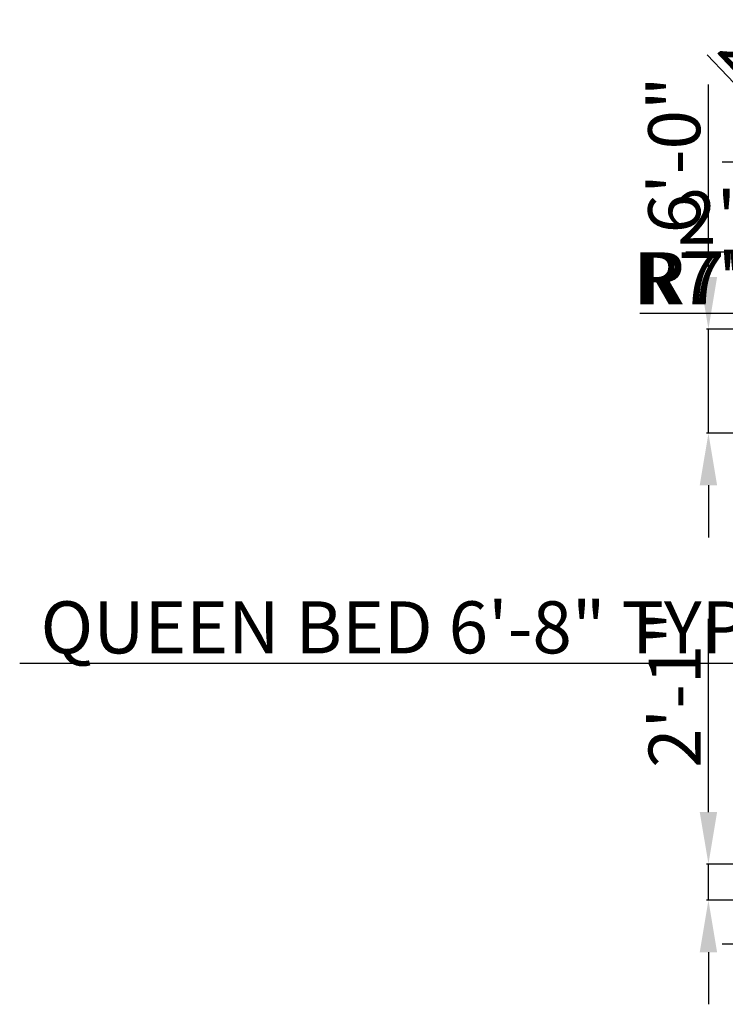
# Model space of a CAD drawing. Units: inches. Extents: x -299 to 1164, y -2 to 940.
# Tile 1 of 11: x -299 to 189, y 86 to 768. Entities that reach past the tile are written whole.
import ezdxf

# ---------------------------------------------------------------- set-up
doc = ezdxf.new("R2010")
doc.units = ezdxf.units.IN
doc.layers.add('dimensions', color=191, linetype='Continuous', lineweight=18)
doc.styles.get("Standard").update_dxf_attribs({"font": 'arial.ttf'})
doc.dimstyles.new('ISO-25', dxfattribs={"dimtxt": 36, "dimasz": 36, "dimexe": 1.25, "dimexo": 0.625, "dimtad": 1, "dimlunit": 3, "dimtxsty": 'Standard', "dimcen": 2.5, "dimazin": 0, "dimtfac": 1, "dimtmove": 0, "dimatfit": 3, "dimfxl": 1, "dimarcsym": 0})

# ---------------------------------------------------------------- blocks, each defined once
blk = doc.blocks.new('*D26')
at = {"layer": 'Defpoints', "color": 0, "transparency": 16777216}
for p in [(415.32, 606.83), (415.32, 597.1), (443.65, 597.1)]:
    blk.add_point(p, dxfattribs=at)
at = {"layer": 'dimensions', "color": 0, "lineweight": -2, "transparency": 16777216}
for p, q in [((379.32, 606.83), (161.88, 606.83)), ((415.32, 597.72), (415.32, 608.08)), ((443.65, 606.83), (415.32, 606.83)), ((443.65, 597.72), (443.65, 608.08)), ((479.65, 606.83), (515.65, 606.83))]:
    blk.add_line(p, q, dxfattribs=at)
at = {"layer": 'dimensions', "color": 0, "transparency": 16777216}
for points in [[(379.32, 612.83), (379.32, 600.83), (415.32, 606.83)], [(479.65, 612.83), (479.65, 600.83), (443.65, 606.83)]]:
    blk.add_solid(points, dxfattribs=at)
at = {"layer": 'dimensions', "color": 0, "transparency": 16777216, "insert": (252.6, 626.07), "char_height": 36, "attachment_point": 5}
blk.add_mtext('2\'-4 1/2"', dxfattribs=at)
blk = doc.blocks.new('*D31')
at = {"layer": 'Defpoints', "color": 0, "transparency": 16777216}
for p in [(268.07, 322.2), (268.07, 310.2), (348.07, 310.2)]:
    blk.add_point(p, dxfattribs=at)
at = {"layer": 'dimensions', "color": 0, "lineweight": -2, "transparency": 16777216}
for p, q in [((268.07, 322.2), (-298.74, 322.2)), ((268.07, 310.83), (268.07, 323.45)), ((312.07, 322.2), (304.07, 322.2)), ((348.07, 310.83), (348.07, 323.45))]:
    blk.add_line(p, q, dxfattribs=at)
at = {"layer": 'dimensions', "color": 0, "transparency": 16777216}
for points in [[(304.07, 328.2), (304.07, 316.2), (268.07, 322.2)], [(312.07, 328.2), (312.07, 316.2), (348.07, 322.2)]]:
    blk.add_solid(points, dxfattribs=at)
at = {"layer": 'dimensions', "color": 0, "transparency": 16777216, "insert": (-33.34, 342.55), "char_height": 36, "attachment_point": 5}
blk.add_mtext('QUEEN BED 6\'-8" TYP.', dxfattribs=at)
blk = doc.blocks.new('*D43')
at = {"layer": 'Defpoints', "color": 0, "transparency": 16777216}
for p in [(268.07, 668.99), (259.07, 638.49), (268.07, 629.49)]:
    blk.add_point(p, dxfattribs=at)
at = {"layer": 'dimensions', "color": 0, "lineweight": -2, "transparency": 16777216}
for p, q in [((223.07, 668.99), (187.07, 668.99)), ((259.07, 639.11), (259.07, 670.24)), ((259.07, 668.99), (268.07, 668.99)), ((268.07, 630.11), (268.07, 670.24)), ((304.07, 668.99), (437.02, 668.99))]:
    blk.add_line(p, q, dxfattribs=at)
at = {"layer": 'dimensions', "color": 0, "transparency": 16777216}
for points in [[(223.07, 674.99), (223.07, 662.99), (259.07, 668.99)], [(304.07, 674.99), (304.07, 662.99), (268.07, 668.99)]]:
    blk.add_solid(points, dxfattribs=at)
at = {"layer": 'dimensions', "color": 0, "transparency": 16777216, "insert": (388.54, 687.99), "char_height": 36, "attachment_point": 5}
blk.add_mtext('0\'-9"', dxfattribs=at)
blk = doc.blocks.new('*D49')
at = {"layer": 'Defpoints', "color": 0, "transparency": 16777216}
for p in [(259.07, 183.49), (304.07, 183.49), (304.07, 127.99)]:
    blk.add_point(p, dxfattribs=at)
at = {"layer": 'dimensions', "color": 0, "lineweight": -2, "transparency": 16777216}
for p, q in [((259.07, 182.86), (259.07, 126.74)), ((304.07, 182.86), (304.07, 126.74)), ((223.07, 127.99), (187.07, 127.99)), ((259.07, 127.99), (304.07, 127.99)), ((340.07, 127.99), (472.99, 127.99))]:
    blk.add_line(p, q, dxfattribs=at)
at = {"layer": 'dimensions', "color": 0, "transparency": 16777216}
for points in [[(223.07, 133.99), (223.07, 121.99), (259.07, 127.99)], [(340.07, 133.99), (340.07, 121.99), (304.07, 127.99)]]:
    blk.add_solid(points, dxfattribs=at)
at = {"layer": 'dimensions', "color": 0, "transparency": 16777216, "insert": (424.53, 147.01), "char_height": 36, "attachment_point": 5}
blk.add_mtext('3\'-9"', dxfattribs=at)
blk = doc.blocks.new('*D50')
at = {"layer": 'Defpoints', "color": 0, "transparency": 16777216}
for p in [(177.57, 183.49), (259.07, 183.49), (259.07, 158.49)]:
    blk.add_point(p, dxfattribs=at)
at = {"layer": 'dimensions', "color": 0, "lineweight": -2, "transparency": 16777216}
for p, q in [((177.57, 219.49), (177.57, 353.05)), ((258.45, 183.49), (176.32, 183.49)), ((177.57, 158.49), (177.57, 183.49)), ((258.45, 158.49), (176.32, 158.49)), ((177.57, 122.49), (177.57, 86.49))]:
    blk.add_line(p, q, dxfattribs=at)
at = {"layer": 'dimensions', "color": 0, "transparency": 16777216}
for points in [[(171.57, 219.49), (183.57, 219.49), (177.57, 183.49)], [(171.57, 122.49), (183.57, 122.49), (177.57, 158.49)]]:
    blk.add_solid(points, dxfattribs=at)
at = {"layer": 'dimensions', "color": 0, "transparency": 16777216, "insert": (158.87, 304.27), "char_height": 36, "attachment_point": 5, "rotation": 90}
blk.add_mtext('2\'-1"', dxfattribs=at)
blk = doc.blocks.new('*D53')
at = {"layer": 'Defpoints', "color": 0, "transparency": 16777216}
for p in [(177.57, 553.49), (586.07, 553.49), (586.07, 481.49)]:
    blk.add_point(p, dxfattribs=at)
at = {"layer": 'dimensions', "color": 0, "lineweight": -2, "transparency": 16777216}
for p, q in [((177.57, 589.49), (177.57, 722.63)), ((585.45, 553.49), (176.32, 553.49)), ((177.57, 481.49), (177.57, 553.49)), ((585.45, 481.49), (176.32, 481.49)), ((177.57, 445.49), (177.57, 409.49))]:
    blk.add_line(p, q, dxfattribs=at)
at = {"layer": 'dimensions', "color": 0, "transparency": 16777216}
for points in [[(171.57, 589.49), (183.57, 589.49), (177.57, 553.49)], [(171.57, 445.49), (183.57, 445.49), (177.57, 481.49)]]:
    blk.add_solid(points, dxfattribs=at)
at = {"layer": 'dimensions', "color": 0, "transparency": 16777216, "insert": (158.57, 674.06), "char_height": 36, "attachment_point": 5, "rotation": 90}
blk.add_mtext('6\'-0"', dxfattribs=at)
blk = doc.blocks.new('*D61')
at = {"layer": 'Defpoints', "color": 0, "transparency": 16777216}
for p in [(389.15, 518.35), (412.32, 493.81)]:
    blk.add_point(p, dxfattribs=at)
at = {"layer": 'dimensions', "color": 0, "lineweight": -2, "transparency": 16777216}
for p, q in [((176.74, 743.24), (364.43, 544.52)), ((412.32, 493.81), (389.15, 518.35))]:
    blk.add_line(p, q, dxfattribs=at)
at = {"layer": 'dimensions', "color": 0, "transparency": 16777216}
blk.add_solid([(368.79, 548.64), (360.07, 540.4), (389.15, 518.35)], dxfattribs=at)
at = {"layer": 'dimensions', "color": 0, "transparency": 16777216, "insert": (272.04, 670.02), "char_height": 36, "attachment_point": 5, "rotation": 313.36444}
blk.add_mtext('2X R2\'-10"', dxfattribs=at)
blk = doc.blocks.new('*D68')
at = {"layer": 'Defpoints', "color": 0, "transparency": 16777216}
for p in [(422.02, 564.66), (515.63, 564.66)]:
    blk.add_point(p, dxfattribs=at)
at = {"layer": 'dimensions', "color": 0, "lineweight": -2, "transparency": 16777216}
for p, q in [((134.73, 564.66), (386.02, 564.66)), ((515.63, 564.66), (422.02, 564.66))]:
    blk.add_line(p, q, dxfattribs=at)
at = {"layer": 'dimensions', "color": 0, "transparency": 16777216}
blk.add_solid([(386.02, 570.66), (386.02, 558.66), (422.02, 564.66)], dxfattribs=at)
at = {"layer": 'dimensions', "color": 0, "transparency": 16777216, "insert": (242.37, 583.9), "char_height": 36, "attachment_point": 5, "rotation": 359.99973}
blk.add_mtext('R7\'-9 1/2"', dxfattribs=at)
blk = doc.blocks.new('*D70')
at = {"layer": 'Defpoints', "color": 0, "transparency": 16777216}
for p in [(417.38, 564.66), (505.63, 564.66)]:
    blk.add_point(p, dxfattribs=at)
at = {"layer": 'dimensions', "color": 0, "lineweight": -2, "transparency": 16777216}
for p, q in [((130.1, 564.66), (381.38, 564.66)), ((505.63, 564.66), (417.38, 564.66))]:
    blk.add_line(p, q, dxfattribs=at)
at = {"layer": 'dimensions', "color": 0, "transparency": 16777216}
blk.add_solid([(381.38, 570.66), (381.38, 558.66), (417.38, 564.66)], dxfattribs=at)
at = {"layer": 'dimensions', "color": 0, "transparency": 16777216, "insert": (237.74, 583.9), "char_height": 36, "attachment_point": 5, "rotation": 359.99972}
blk.add_mtext('R7\'-4 1/2"', dxfattribs=at)

msp = doc.modelspace()

# ---------------------------------------------------------------- dimensions: what is measured, and where the dimension line sits
at = {"layer": 'dimensions'}
dim = msp.add_radius_dim(center=(412.321, 493.813), mpoint=(389.146, 518.35), text='2X <>', dimstyle='ISO-25', override={"dimdec": 1, "dimlfac": 1, "dimrnd": 0, "dimzin": 1, "dimdsep": 46, "dimlunit": 4, "dimfrac": 2}, dxfattribs=at)
dim.commit()
dim.dimension.update_dxf_attribs({"geometry": '*D61', "text_midpoint": (272.043, 670.016)})
for base, p1, p2, angle, picture, middle in [((177.571, 553.489), (586.071, 481.489), (586.071, 553.489), 90, '*D53', (158.565, 674.061)), ((415.323, 606.831), (443.646, 597.099), (415.323, 597.099), 180, '*D26', (252.6, 626.07)), ((177.571, 183.489), (259.071, 158.489), (259.071, 183.489), 90, '*D50', (158.872, 304.27))]:
    dim = msp.add_linear_dim(base=base, p1=p1, p2=p2, angle=angle, dimstyle='ISO-25', override={"dimdec": 1, "dimlfac": 1, "dimrnd": 0, "dimzin": 1, "dimdsep": 46, "dimlunit": 4, "dimfrac": 2}, dxfattribs=at)
    dim.commit()
    dim.dimension.update_dxf_attribs({"geometry": picture, "text_midpoint": middle})
for base, p1, p2, picture, middle in [((268.071, 668.989), (259.071, 638.489), (268.071, 629.489), '*D43', (388.545, 687.995)), ((304.071, 127.989), (259.071, 183.489), (304.071, 183.489), '*D49', (424.532, 147.007))]:
    dim = msp.add_linear_dim(base=base, p1=p1, p2=p2, dimstyle='ISO-25', override={"dimdec": 1, "dimlfac": 1, "dimrnd": 0, "dimzin": 1, "dimdsep": 46, "dimlunit": 4, "dimfrac": 2}, dxfattribs=at)
    dim.commit()
    dim.dimension.update_dxf_attribs({"geometry": picture, "text_midpoint": middle})
for center, mpoint, picture, middle in [((505.6333, 564.6566), (417.383, 564.657), '*D70', (237.7404, 583.8968)), ((515.634, 564.657), (422.018, 564.657), '*D68', (242.375, 583.897))]:
    dim = msp.add_radius_dim(center=center, mpoint=mpoint, dimstyle='ISO-25', override={"dimdec": 1, "dimlfac": 1, "dimrnd": 0, "dimzin": 1, "dimdsep": 46, "dimlunit": 4, "dimfrac": 2}, dxfattribs=at)
    dim.commit()
    dim.dimension.update_dxf_attribs({"geometry": picture, "text_midpoint": middle})
dim = msp.add_linear_dim(base=(268.071, 322.202), p1=(348.071, 310.202), p2=(268.071, 310.202), angle=180, text='QUEEN BED <> TYP.', dimstyle='ISO-25', override={"dimdec": 1, "dimlfac": 1, "dimrnd": 0, "dimzin": 1, "dimdsep": 46, "dimlunit": 4, "dimfrac": 2}, dxfattribs=at)
dim.commit()
dim.dimension.update_dxf_attribs({"geometry": '*D31', "text_midpoint": (-33.336, 342.546)})

doc.saveas('drawing.dxf')
